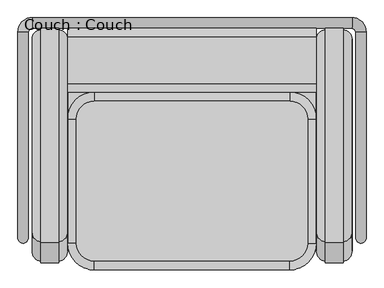
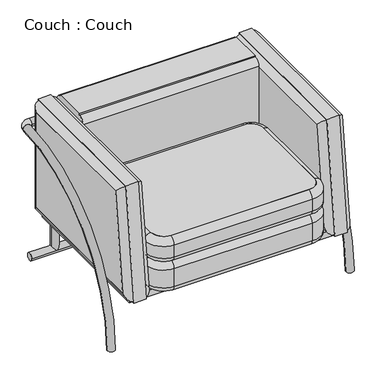
"""IFC4 building model written with IfcOpenShell, lengths in millimetres: furniture geometry, Couch : Couch."""

from ifc_helpers import new_model, si_unit, point, frame, frame_2d, origin, place, context, project, spatial, polyline, circle_curve, ellipse_curve, trimmed, segment, composite_curve, outline, extrude, source, transform, mapped, element, save
from ifc_brep_helpers import plane_surface, cylinder_surface, revolved_surface, advanced_brep


def couch_couch_04099933(model_context):
    return source(origin(), model_context, "Body", "SolidModel", [
        extrude(outline(composite_curve([segment(trimmed(circle_curve(frame_2d((275.0, 175.0)), 50.0), [point((275.0, 225.0))], [point((325.0, 175.0))], False, "CARTESIAN"), True, "CONTINUOUS"), segment(polyline([(325.0, 175.0), (325.0, -175.0)]), True, "CONTINUOUS"), segment(trimmed(circle_curve(frame_2d((275.0, -175.0)), 50.0), [point((325.0, -175.0))], [point((275.0, -225.0))], False, "CARTESIAN"), True, "CONTINUOUS"), segment(polyline([(275.0, -225.0), (-275.0, -225.0)]), True, "CONTINUOUS"), segment(trimmed(circle_curve(frame_2d((-275.0, -175.0)), 50.0), [point((-275.0, -225.0))], [point((-325.0, -175.0))], False, "CARTESIAN"), True, "CONTINUOUS"), segment(polyline([(-325.0, -175.0), (-325.0, 175.0)]), True, "CONTINUOUS"), segment(trimmed(circle_curve(frame_2d((-275.0, 175.0)), 50.0), [point((-325.0, 175.0))], [point((-275.0, 225.0))], False, "CARTESIAN"), True, "CONTINUOUS"), segment(polyline([(-275.0, 225.0), (275.0, 225.0)]), True, "CONTINUOUS")], self_intersect=False)), frame((0.0, 0.0, 350.0), z_axis=(0.0, 0.0, 1.0), x_axis=(1.0, 0.0, 0.0)), (0.0, 0.0, 1.0), 100.0),
        advanced_brep(
        [(-275.0, 225.0, 450.0), (-325.0, 175.0, 450.0), (-325.0, 175.0, 350.0), (-275.0, 225.0, 350.0), (-275.0, 250.0, 425.0), (-350.0, 175.0, 425.0), (-275.0, 250.0, 375.0), (-350.0, 175.0, 375.0), (275.0, 225.0, 350.0), (275.0, 225.0, 450.0), (275.0, 250.0, 425.0), (275.0, 250.0, 375.0), (325.0, 175.0, 450.0), (325.0, 175.0, 350.0), (350.0, 175.0, 425.0), (350.0, 175.0, 375.0), (325.0, -175.0, 350.0), (325.0, -175.0, 450.0), (350.0, -175.0, 425.0), (350.0, -175.0, 375.0), (275.0, -225.0, 450.0), (275.0, -225.0, 350.0), (275.0, -250.0, 425.0), (275.0, -250.0, 375.0), (-275.0, -225.0, 350.0), (-275.0, -225.0, 450.0), (-275.0, -250.0, 425.0), (-275.0, -250.0, 375.0), (-325.0, -175.0, 450.0), (-325.0, -175.0, 350.0), (-350.0, -175.0, 425.0), (-350.0, -175.0, 375.0)],
        [
            (0, 1, circle_curve(frame((-275.0, 175.0, 450.0), z_axis=(0.0, 0.0, 1.0), x_axis=(-1.0, 0.0, 0.0)), 50.0)),
            (1, 2),
            (2, 3, circle_curve(frame((-275.0, 175.0, 350.0), z_axis=(0.0, 0.0, -1.0), x_axis=(-1.0, 0.0, 0.0)), 50.0)),
            (3, 0),
            (4, 5, circle_curve(frame((-275.0, 175.0, 425.0), z_axis=(0.0, 0.0, 1.0), x_axis=(-1.0, 0.0, 0.0)), 75.0)),
            (5, 1, circle_curve(frame((-325.0, 175.0, 425.0), z_axis=(0.0, 1.0, 0.0), x_axis=(1.0, 0.0, 0.0)), 25.0)),
            (0, 4, circle_curve(frame((-275.0, 225.0, 425.0), z_axis=(-1.0, 0.0, 0.0), x_axis=(0.0, -1.0, 0.0)), 25.0)),
            (6, 7, circle_curve(frame((-275.0, 175.0, 375.0), z_axis=(0.0, 0.0, 1.0), x_axis=(-1.0, 0.0, 0.0)), 75.0)),
            (7, 5),
            (4, 6),
            (2, 7, circle_curve(frame((-325.0, 175.0, 375.0), z_axis=(0.0, 1.0, 0.0), x_axis=(1.0, 0.0, 0.0)), 25.0)),
            (6, 3, circle_curve(frame((-275.0, 225.0, 375.0), z_axis=(-1.0, 0.0, 0.0), x_axis=(0.0, -1.0, 0.0)), 25.0)),
            (3, 8),
            (8, 9),
            (9, 0),
            (9, 10, circle_curve(frame((275.0, 225.0, 425.0), z_axis=(-1.0, 0.0, 0.0), x_axis=(0.0, -1.0, 0.0)), 25.0)),
            (10, 4),
            (10, 11),
            (11, 6),
            (11, 8, circle_curve(frame((275.0, 225.0, 375.0), z_axis=(-1.0, 0.0, 0.0), x_axis=(0.0, -1.0, 0.0)), 25.0)),
            (12, 9, circle_curve(frame((275.0, 175.0, 450.0), z_axis=(0.0, 0.0, 1.0), x_axis=(0.0, 1.0, 0.0)), 50.0)),
            (8, 13, circle_curve(frame((275.0, 175.0, 350.0), z_axis=(0.0, 0.0, -1.0), x_axis=(0.0, 1.0, 0.0)), 50.0)),
            (13, 12),
            (14, 10, circle_curve(frame((275.0, 175.0, 425.0), z_axis=(0.0, 0.0, 1.0), x_axis=(0.0, 1.0, 0.0)), 75.0)),
            (12, 14, circle_curve(frame((325.0, 175.0, 425.0), z_axis=(0.0, 1.0, 0.0), x_axis=(-1.0, 0.0, 0.0)), 25.0)),
            (15, 11, circle_curve(frame((275.0, 175.0, 375.0), z_axis=(0.0, 0.0, 1.0), x_axis=(0.0, 1.0, 0.0)), 75.0)),
            (14, 15),
            (15, 13, circle_curve(frame((325.0, 175.0, 375.0), z_axis=(0.0, 1.0, 0.0), x_axis=(-1.0, 0.0, 0.0)), 25.0)),
            (13, 16),
            (16, 17),
            (17, 12),
            (17, 18, circle_curve(frame((325.0, -175.0, 425.0), z_axis=(0.0, 1.0, 0.0), x_axis=(-1.0, 0.0, 0.0)), 25.0)),
            (18, 14),
            (18, 19),
            (19, 15),
            (19, 16, circle_curve(frame((325.0, -175.0, 375.0), z_axis=(0.0, 1.0, 0.0), x_axis=(-1.0, 0.0, 0.0)), 25.0)),
            (20, 17, circle_curve(frame((275.0, -175.0, 450.0), z_axis=(0.0, 0.0, 1.0), x_axis=(1.0, 0.0, 0.0)), 50.0)),
            (16, 21, circle_curve(frame((275.0, -175.0, 350.0), z_axis=(0.0, 0.0, -1.0), x_axis=(1.0, 0.0, 0.0)), 50.0)),
            (21, 20),
            (22, 18, circle_curve(frame((275.0, -175.0, 425.0), z_axis=(0.0, 0.0, 1.0), x_axis=(1.0, 0.0, 0.0)), 75.0)),
            (20, 22, circle_curve(frame((275.0, -225.0, 425.0), z_axis=(1.0, 0.0, 0.0), x_axis=(0.0, 1.0, 0.0)), 25.0)),
            (23, 19, circle_curve(frame((275.0, -175.0, 375.0), z_axis=(0.0, 0.0, 1.0), x_axis=(1.0, 0.0, 0.0)), 75.0)),
            (22, 23),
            (23, 21, circle_curve(frame((275.0, -225.0, 375.0), z_axis=(1.0, 0.0, 0.0), x_axis=(0.0, 1.0, 0.0)), 25.0)),
            (21, 24),
            (24, 25),
            (25, 20),
            (25, 26, circle_curve(frame((-275.0, -225.0, 425.0), z_axis=(1.0, 0.0, 0.0), x_axis=(0.0, 1.0, 0.0)), 25.0)),
            (26, 22),
            (26, 27),
            (27, 23),
            (27, 24, circle_curve(frame((-275.0, -225.0, 375.0), z_axis=(1.0, 0.0, 0.0), x_axis=(0.0, 1.0, 0.0)), 25.0)),
            (28, 25, circle_curve(frame((-275.0, -175.0, 450.0), z_axis=(0.0, 0.0, 1.0), x_axis=(0.0, -1.0, 0.0)), 50.0)),
            (24, 29, circle_curve(frame((-275.0, -175.0, 350.0), z_axis=(0.0, 0.0, -1.0), x_axis=(0.0, -1.0, 0.0)), 50.0)),
            (29, 28),
            (30, 26, circle_curve(frame((-275.0, -175.0, 425.0), z_axis=(0.0, 0.0, 1.0), x_axis=(0.0, -1.0, 0.0)), 75.0)),
            (28, 30, circle_curve(frame((-325.0, -175.0, 425.0), z_axis=(0.0, -1.0, 0.0), x_axis=(1.0, 0.0, 0.0)), 25.0)),
            (31, 27, circle_curve(frame((-275.0, -175.0, 375.0), z_axis=(0.0, 0.0, 1.0), x_axis=(0.0, -1.0, 0.0)), 75.0)),
            (30, 31),
            (31, 29, circle_curve(frame((-325.0, -175.0, 375.0), z_axis=(0.0, -1.0, 0.0), x_axis=(1.0, 0.0, 0.0)), 25.0)),
            (29, 2),
            (1, 28),
            (5, 30),
            (7, 31),
        ],
        [
            revolved_surface(polyline([(-325.0, 175.0, 350.0), (-325.0, 175.0, 450.0)]), (-275.0, 175.0, 0.0), (0.0, 0.0, -1.0)),
            revolved_surface(trimmed(ellipse_curve(frame((-325.0, 175.0, 425.0), z_axis=(0.0, -1.0, 0.0), x_axis=(1.0, 0.0, 0.0)), 25.0, 25.0), [point((-325.0, 175.0, 450.0))], [point((-350.0, 175.0, 425.0))], True, "CARTESIAN"), (-275.0, 175.0, 0.0), (0.0, 0.0, -1.0)),
            cylinder_surface(frame((-275.0, 175.0, 0.0), z_axis=(0.0, 0.0, -1.0), x_axis=(-1.0, 0.0, 0.0)), 75.0),
            revolved_surface(trimmed(ellipse_curve(frame((-325.0, 175.0, 375.0), z_axis=(0.0, -1.0, 0.0), x_axis=(1.0, 0.0, 0.0)), 25.0, 25.0), [point((-350.0, 175.0, 375.0))], [point((-325.0, 175.0, 350.0))], True, "CARTESIAN"), (-275.0, 175.0, 0.0), (0.0, 0.0, -1.0)),
            plane_surface(frame((-275.0, 225.0, 350.0), z_axis=(0.0, -1.0, 0.0), x_axis=(1.0, 0.0, 0.0))),
            cylinder_surface(frame((-275.0, 225.0, 425.0), z_axis=(-1.0, 0.0, 0.0), x_axis=(0.0, -1.0, 0.0)), 25.0),
            plane_surface(frame((-275.0, 250.0, 425.0), z_axis=(0.0, 1.0, 0.0), x_axis=(1.0, 0.0, 0.0))),
            cylinder_surface(frame((-275.0, 225.0, 375.0), z_axis=(-1.0, 0.0, 0.0), x_axis=(0.0, -1.0, 0.0)), 25.0),
            revolved_surface(polyline([(275.0, 225.0, 350.0), (275.0, 225.0, 450.0)]), (275.0, 175.0, 0.0), (0.0, 0.0, -1.0)),
            revolved_surface(trimmed(ellipse_curve(frame((275.0, 225.0, 425.0), z_axis=(-1.0, 0.0, 0.0), x_axis=(0.0, -1.0, 0.0)), 25.0, 25.0), [point((275.0, 225.0, 450.0))], [point((275.0, 250.0, 425.0))], True, "CARTESIAN"), (275.0, 175.0, 0.0), (0.0, 0.0, -1.0)),
            cylinder_surface(frame((275.0, 175.0, 0.0), z_axis=(0.0, 0.0, -1.0), x_axis=(0.0, 1.0, 0.0)), 75.0),
            revolved_surface(trimmed(ellipse_curve(frame((275.0, 225.0, 375.0), z_axis=(-1.0, 0.0, 0.0), x_axis=(0.0, -1.0, 0.0)), 25.0, 25.0), [point((275.0, 250.0, 375.0))], [point((275.0, 225.0, 350.0))], True, "CARTESIAN"), (275.0, 175.0, 0.0), (0.0, 0.0, -1.0)),
            plane_surface(frame((325.0, 175.0, 350.0), z_axis=(-1.0, 0.0, 0.0), x_axis=(0.0, -1.0, 0.0))),
            cylinder_surface(frame((325.0, 175.0, 425.0), z_axis=(0.0, 1.0, 0.0), x_axis=(-1.0, 0.0, 0.0)), 25.0),
            plane_surface(frame((350.0, 175.0, 425.0), z_axis=(1.0, 0.0, 0.0), x_axis=(0.0, -1.0, 0.0))),
            cylinder_surface(frame((325.0, 175.0, 375.0), z_axis=(0.0, 1.0, 0.0), x_axis=(-1.0, 0.0, 0.0)), 25.0),
            revolved_surface(polyline([(325.0, -175.0, 350.0), (325.0, -175.0, 450.0)]), (275.0, -175.0, 0.0), (0.0, 0.0, -1.0)),
            revolved_surface(trimmed(ellipse_curve(frame((325.0, -175.0, 425.0), z_axis=(0.0, 1.0, 0.0), x_axis=(-1.0, 0.0, 0.0)), 25.0, 25.0), [point((325.0, -175.0, 450.0))], [point((350.0, -175.0, 425.0))], True, "CARTESIAN"), (275.0, -175.0, 0.0), (0.0, 0.0, -1.0)),
            cylinder_surface(frame((275.0, -175.0, 0.0), z_axis=(0.0, 0.0, -1.0), x_axis=(1.0, 0.0, 0.0)), 75.0),
            revolved_surface(trimmed(ellipse_curve(frame((325.0, -175.0, 375.0), z_axis=(0.0, 1.0, 0.0), x_axis=(-1.0, 0.0, 0.0)), 25.0, 25.0), [point((350.0, -175.0, 375.0))], [point((325.0, -175.0, 350.0))], True, "CARTESIAN"), (275.0, -175.0, 0.0), (0.0, 0.0, -1.0)),
            plane_surface(frame((275.0, -225.0, 350.0), z_axis=(0.0, 1.0, 0.0), x_axis=(-1.0, 0.0, 0.0))),
            cylinder_surface(frame((275.0, -225.0, 425.0), z_axis=(1.0, 0.0, 0.0), x_axis=(0.0, 1.0, 0.0)), 25.0),
            plane_surface(frame((275.0, -250.0, 425.0), z_axis=(0.0, -1.0, 0.0), x_axis=(-1.0, 0.0, 0.0))),
            cylinder_surface(frame((275.0, -225.0, 375.0), z_axis=(1.0, 0.0, 0.0), x_axis=(0.0, 1.0, 0.0)), 25.0),
            revolved_surface(polyline([(-275.0, -225.0, 350.0), (-275.0, -225.0, 450.0)]), (-275.0, -175.0, 0.0), (0.0, 0.0, -1.0)),
            revolved_surface(trimmed(ellipse_curve(frame((-275.0, -225.0, 425.0), z_axis=(1.0, 0.0, 0.0), x_axis=(0.0, 1.0, 0.0)), 25.0, 25.0), [point((-275.0, -225.0, 450.0))], [point((-275.0, -250.0, 425.0))], True, "CARTESIAN"), (-275.0, -175.0, 0.0), (0.0, 0.0, -1.0)),
            cylinder_surface(frame((-275.0, -175.0, 0.0), z_axis=(0.0, 0.0, -1.0), x_axis=(0.0, -1.0, 0.0)), 75.0),
            revolved_surface(trimmed(ellipse_curve(frame((-275.0, -225.0, 375.0), z_axis=(1.0, 0.0, 0.0), x_axis=(0.0, 1.0, 0.0)), 25.0, 25.0), [point((-275.0, -250.0, 375.0))], [point((-275.0, -225.0, 350.0))], True, "CARTESIAN"), (-275.0, -175.0, 0.0), (0.0, 0.0, -1.0)),
            plane_surface(frame((-325.0, -175.0, 350.0), z_axis=(1.0, 0.0, 0.0), x_axis=(0.0, 1.0, 0.0))),
            cylinder_surface(frame((-325.0, -175.0, 425.0), z_axis=(0.0, -1.0, 0.0), x_axis=(1.0, 0.0, 0.0)), 25.0),
            plane_surface(frame((-350.0, -175.0, 425.0), z_axis=(-1.0, 0.0, 0.0), x_axis=(0.0, 1.0, 0.0))),
            cylinder_surface(frame((-325.0, -175.0, 375.0), z_axis=(0.0, -1.0, 0.0), x_axis=(1.0, 0.0, 0.0)), 25.0),
        ],
        [
            (0, [[1, 2, 3, 4]]),
            (1, [[5, 6, -1, 7]]),
            (2, [[8, 9, -5, 10]]),
            (3, [[-3, 11, -8, 12]]),
            (4, [[-4, 13, 14, 15]]),
            (5, [[-7, -15, 16, 17]]),
            (6, [[-10, -17, 18, 19]]),
            (7, [[-12, -19, 20, -13]]),
            (8, [[21, -14, 22, 23]]),
            (9, [[24, -16, -21, 25]]),
            (10, [[26, -18, -24, 27]]),
            (11, [[-22, -20, -26, 28]]),
            (12, [[-23, 29, 30, 31]]),
            (13, [[-25, -31, 32, 33]]),
            (14, [[-27, -33, 34, 35]]),
            (15, [[-28, -35, 36, -29]]),
            (16, [[37, -30, 38, 39]]),
            (17, [[40, -32, -37, 41]]),
            (18, [[42, -34, -40, 43]]),
            (19, [[-38, -36, -42, 44]]),
            (20, [[-39, 45, 46, 47]]),
            (21, [[-41, -47, 48, 49]]),
            (22, [[-43, -49, 50, 51]]),
            (23, [[-44, -51, 52, -45]]),
            (24, [[53, -46, 54, 55]]),
            (25, [[56, -48, -53, 57]]),
            (26, [[58, -50, -56, 59]]),
            (27, [[-54, -52, -58, 60]]),
            (28, [[-55, 61, -2, 62]]),
            (29, [[-57, -62, -6, 63]]),
            (30, [[-59, -63, -9, 64]]),
            (31, [[-60, -64, -11, -61]]),
        ],
    ),
        advanced_brep(
        [(-275.0, 225.0, 350.0), (-325.0, 175.0, 350.0), (-325.0, 175.0, 225.0), (-275.0, 225.0, 225.0), (-275.0, 250.0, 325.0), (-350.0, 175.0, 325.0), (-275.0, 250.0, 250.0), (-350.0, 175.0, 250.0), (275.0, 225.0, 225.0), (275.0, 225.0, 350.0), (275.0, 250.0, 325.0), (275.0, 250.0, 250.0), (325.0, 175.0, 350.0), (325.0, 175.0, 225.0), (350.0, 175.0, 325.0), (350.0, 175.0, 250.0), (325.0, -175.0, 225.0), (325.0, -175.0, 350.0), (350.0, -175.0, 325.0), (350.0, -175.0, 250.0), (275.0, -225.0, 350.0), (275.0, -225.0, 225.0), (275.0, -250.0, 325.0), (275.0, -250.0, 250.0), (-275.0, -225.0, 225.0), (-275.0, -225.0, 350.0), (-275.0, -250.0, 325.0), (-275.0, -250.0, 250.0), (-325.0, -175.0, 350.0), (-325.0, -175.0, 225.0), (-350.0, -175.0, 325.0), (-350.0, -175.0, 250.0)],
        [
            (0, 1, circle_curve(frame((-275.0, 175.0, 350.0), z_axis=(0.0, 0.0, 1.0), x_axis=(-1.0, 0.0, 0.0)), 50.0)),
            (1, 2),
            (2, 3, circle_curve(frame((-275.0, 175.0, 225.0), z_axis=(0.0, 0.0, -1.0), x_axis=(-1.0, 0.0, 0.0)), 50.0)),
            (3, 0),
            (4, 5, circle_curve(frame((-275.0, 175.0, 325.0), z_axis=(0.0, 0.0, 1.0), x_axis=(-1.0, 0.0, 0.0)), 75.0)),
            (5, 1, circle_curve(frame((-325.0, 175.0, 325.0), z_axis=(0.0, 1.0, 0.0), x_axis=(1.0, 0.0, 0.0)), 25.0)),
            (0, 4, circle_curve(frame((-275.0, 225.0, 325.0), z_axis=(-1.0, 0.0, 0.0), x_axis=(0.0, -1.0, 0.0)), 25.0)),
            (6, 7, circle_curve(frame((-275.0, 175.0, 250.0), z_axis=(0.0, 0.0, 1.0), x_axis=(-1.0, 0.0, 0.0)), 75.0)),
            (7, 5),
            (4, 6),
            (2, 7, circle_curve(frame((-325.0, 175.0, 250.0), z_axis=(0.0, 1.0, 0.0), x_axis=(1.0, 0.0, 0.0)), 25.0)),
            (6, 3, circle_curve(frame((-275.0, 225.0, 250.0), z_axis=(-1.0, 0.0, 0.0), x_axis=(0.0, -1.0, 0.0)), 25.0)),
            (3, 8),
            (8, 9),
            (9, 0),
            (9, 10, circle_curve(frame((275.0, 225.0, 325.0), z_axis=(-1.0, 0.0, 0.0), x_axis=(0.0, -1.0, 0.0)), 25.0)),
            (10, 4),
            (10, 11),
            (11, 6),
            (11, 8, circle_curve(frame((275.0, 225.0, 250.0), z_axis=(-1.0, 0.0, 0.0), x_axis=(0.0, -1.0, 0.0)), 25.0)),
            (12, 9, circle_curve(frame((275.0, 175.0, 350.0), z_axis=(0.0, 0.0, 1.0), x_axis=(0.0, 1.0, 0.0)), 50.0)),
            (8, 13, circle_curve(frame((275.0, 175.0, 225.0), z_axis=(0.0, 0.0, -1.0), x_axis=(0.0, 1.0, 0.0)), 50.0)),
            (13, 12),
            (14, 10, circle_curve(frame((275.0, 175.0, 325.0), z_axis=(0.0, 0.0, 1.0), x_axis=(0.0, 1.0, 0.0)), 75.0)),
            (12, 14, circle_curve(frame((325.0, 175.0, 325.0), z_axis=(0.0, 1.0, 0.0), x_axis=(-1.0, 0.0, 0.0)), 25.0)),
            (15, 11, circle_curve(frame((275.0, 175.0, 250.0), z_axis=(0.0, 0.0, 1.0), x_axis=(0.0, 1.0, 0.0)), 75.0)),
            (14, 15),
            (15, 13, circle_curve(frame((325.0, 175.0, 250.0), z_axis=(0.0, 1.0, 0.0), x_axis=(-1.0, 0.0, 0.0)), 25.0)),
            (13, 16),
            (16, 17),
            (17, 12),
            (17, 18, circle_curve(frame((325.0, -175.0, 325.0), z_axis=(0.0, 1.0, 0.0), x_axis=(-1.0, 0.0, 0.0)), 25.0)),
            (18, 14),
            (18, 19),
            (19, 15),
            (19, 16, circle_curve(frame((325.0, -175.0, 250.0), z_axis=(0.0, 1.0, 0.0), x_axis=(-1.0, 0.0, 0.0)), 25.0)),
            (20, 17, circle_curve(frame((275.0, -175.0, 350.0), z_axis=(0.0, 0.0, 1.0), x_axis=(1.0, 0.0, 0.0)), 50.0)),
            (16, 21, circle_curve(frame((275.0, -175.0, 225.0), z_axis=(0.0, 0.0, -1.0), x_axis=(1.0, 0.0, 0.0)), 50.0)),
            (21, 20),
            (22, 18, circle_curve(frame((275.0, -175.0, 325.0), z_axis=(0.0, 0.0, 1.0), x_axis=(1.0, 0.0, 0.0)), 75.0)),
            (20, 22, circle_curve(frame((275.0, -225.0, 325.0), z_axis=(1.0, 0.0, 0.0), x_axis=(0.0, 1.0, 0.0)), 25.0)),
            (23, 19, circle_curve(frame((275.0, -175.0, 250.0), z_axis=(0.0, 0.0, 1.0), x_axis=(1.0, 0.0, 0.0)), 75.0)),
            (22, 23),
            (23, 21, circle_curve(frame((275.0, -225.0, 250.0), z_axis=(1.0, 0.0, 0.0), x_axis=(0.0, 1.0, 0.0)), 25.0)),
            (21, 24),
            (24, 25),
            (25, 20),
            (25, 26, circle_curve(frame((-275.0, -225.0, 325.0), z_axis=(1.0, 0.0, 0.0), x_axis=(0.0, 1.0, 0.0)), 25.0)),
            (26, 22),
            (26, 27),
            (27, 23),
            (27, 24, circle_curve(frame((-275.0, -225.0, 250.0), z_axis=(1.0, 0.0, 0.0), x_axis=(0.0, 1.0, 0.0)), 25.0)),
            (28, 25, circle_curve(frame((-275.0, -175.0, 350.0), z_axis=(0.0, 0.0, 1.0), x_axis=(0.0, -1.0, 0.0)), 50.0)),
            (24, 29, circle_curve(frame((-275.0, -175.0, 225.0), z_axis=(0.0, 0.0, -1.0), x_axis=(0.0, -1.0, 0.0)), 50.0)),
            (29, 28),
            (30, 26, circle_curve(frame((-275.0, -175.0, 325.0), z_axis=(0.0, 0.0, 1.0), x_axis=(0.0, -1.0, 0.0)), 75.0)),
            (28, 30, circle_curve(frame((-325.0, -175.0, 325.0), z_axis=(0.0, -1.0, 0.0), x_axis=(1.0, 0.0, 0.0)), 25.0)),
            (31, 27, circle_curve(frame((-275.0, -175.0, 250.0), z_axis=(0.0, 0.0, 1.0), x_axis=(0.0, -1.0, 0.0)), 75.0)),
            (30, 31),
            (31, 29, circle_curve(frame((-325.0, -175.0, 250.0), z_axis=(0.0, -1.0, 0.0), x_axis=(1.0, 0.0, 0.0)), 25.0)),
            (29, 2),
            (1, 28),
            (5, 30),
            (7, 31),
        ],
        [
            revolved_surface(polyline([(-325.0, 175.0, 225.0), (-325.0, 175.0, 350.0)]), (-275.0, 175.0, -75.0), (0.0, 0.0, -1.0)),
            revolved_surface(trimmed(ellipse_curve(frame((-325.0, 175.0, 325.0), z_axis=(0.0, -1.0, 0.0), x_axis=(1.0, 0.0, 0.0)), 25.0, 25.0), [point((-325.0, 175.0, 350.0))], [point((-350.0, 175.0, 325.0))], True, "CARTESIAN"), (-275.0, 175.0, -75.0), (0.0, 0.0, -1.0)),
            cylinder_surface(frame((-275.0, 175.0, -75.0), z_axis=(0.0, 0.0, -1.0), x_axis=(-1.0, 0.0, 0.0)), 75.0),
            revolved_surface(trimmed(ellipse_curve(frame((-325.0, 175.0, 250.0), z_axis=(0.0, -1.0, 0.0), x_axis=(1.0, 0.0, 0.0)), 25.0, 25.0), [point((-350.0, 175.0, 250.0))], [point((-325.0, 175.0, 225.0))], True, "CARTESIAN"), (-275.0, 175.0, -75.0), (0.0, 0.0, -1.0)),
            plane_surface(frame((-275.0, 225.0, 225.0), z_axis=(0.0, -1.0, 0.0), x_axis=(1.0, 0.0, 0.0))),
            cylinder_surface(frame((-275.0, 225.0, 325.0), z_axis=(-1.0, 0.0, 0.0), x_axis=(0.0, -1.0, 0.0)), 25.0),
            plane_surface(frame((-275.0, 250.0, 325.0), z_axis=(0.0, 1.0, 0.0), x_axis=(1.0, 0.0, 0.0))),
            cylinder_surface(frame((-275.0, 225.0, 250.0), z_axis=(-1.0, 0.0, 0.0), x_axis=(0.0, -1.0, 0.0)), 25.0),
            revolved_surface(polyline([(275.0, 225.0, 225.0), (275.0, 225.0, 350.0)]), (275.0, 175.0, -75.0), (0.0, 0.0, -1.0)),
            revolved_surface(trimmed(ellipse_curve(frame((275.0, 225.0, 325.0), z_axis=(-1.0, 0.0, 0.0), x_axis=(0.0, -1.0, 0.0)), 25.0, 25.0), [point((275.0, 225.0, 350.0))], [point((275.0, 250.0, 325.0))], True, "CARTESIAN"), (275.0, 175.0, -75.0), (0.0, 0.0, -1.0)),
            cylinder_surface(frame((275.0, 175.0, -75.0), z_axis=(0.0, 0.0, -1.0), x_axis=(0.0, 1.0, 0.0)), 75.0),
            revolved_surface(trimmed(ellipse_curve(frame((275.0, 225.0, 250.0), z_axis=(-1.0, 0.0, 0.0), x_axis=(0.0, -1.0, 0.0)), 25.0, 25.0), [point((275.0, 250.0, 250.0))], [point((275.0, 225.0, 225.0))], True, "CARTESIAN"), (275.0, 175.0, -75.0), (0.0, 0.0, -1.0)),
            plane_surface(frame((325.0, 175.0, 225.0), z_axis=(-1.0, 0.0, 0.0), x_axis=(0.0, -1.0, 0.0))),
            cylinder_surface(frame((325.0, 175.0, 325.0), z_axis=(0.0, 1.0, 0.0), x_axis=(-1.0, 0.0, 0.0)), 25.0),
            plane_surface(frame((350.0, 175.0, 325.0), z_axis=(1.0, 0.0, 0.0), x_axis=(0.0, -1.0, 0.0))),
            cylinder_surface(frame((325.0, 175.0, 250.0), z_axis=(0.0, 1.0, 0.0), x_axis=(-1.0, 0.0, 0.0)), 25.0),
            revolved_surface(polyline([(325.0, -175.0, 225.0), (325.0, -175.0, 350.0)]), (275.0, -175.0, -75.0), (0.0, 0.0, -1.0)),
            revolved_surface(trimmed(ellipse_curve(frame((325.0, -175.0, 325.0), z_axis=(0.0, 1.0, 0.0), x_axis=(-1.0, 0.0, 0.0)), 25.0, 25.0), [point((325.0, -175.0, 350.0))], [point((350.0, -175.0, 325.0))], True, "CARTESIAN"), (275.0, -175.0, -75.0), (0.0, 0.0, -1.0)),
            cylinder_surface(frame((275.0, -175.0, -75.0), z_axis=(0.0, 0.0, -1.0), x_axis=(1.0, 0.0, 0.0)), 75.0),
            revolved_surface(trimmed(ellipse_curve(frame((325.0, -175.0, 250.0), z_axis=(0.0, 1.0, 0.0), x_axis=(-1.0, 0.0, 0.0)), 25.0, 25.0), [point((350.0, -175.0, 250.0))], [point((325.0, -175.0, 225.0))], True, "CARTESIAN"), (275.0, -175.0, -75.0), (0.0, 0.0, -1.0)),
            plane_surface(frame((275.0, -225.0, 225.0), z_axis=(0.0, 1.0, 0.0), x_axis=(-1.0, 0.0, 0.0))),
            cylinder_surface(frame((275.0, -225.0, 325.0), z_axis=(1.0, 0.0, 0.0), x_axis=(0.0, 1.0, 0.0)), 25.0),
            plane_surface(frame((275.0, -250.0, 325.0), z_axis=(0.0, -1.0, 0.0), x_axis=(-1.0, 0.0, 0.0))),
            cylinder_surface(frame((275.0, -225.0, 250.0), z_axis=(1.0, 0.0, 0.0), x_axis=(0.0, 1.0, 0.0)), 25.0),
            revolved_surface(polyline([(-275.0, -225.0, 225.0), (-275.0, -225.0, 350.0)]), (-275.0, -175.0, -75.0), (0.0, 0.0, -1.0)),
            revolved_surface(trimmed(ellipse_curve(frame((-275.0, -225.0, 325.0), z_axis=(1.0, 0.0, 0.0), x_axis=(0.0, 1.0, 0.0)), 25.0, 25.0), [point((-275.0, -225.0, 350.0))], [point((-275.0, -250.0, 325.0))], True, "CARTESIAN"), (-275.0, -175.0, -75.0), (0.0, 0.0, -1.0)),
            cylinder_surface(frame((-275.0, -175.0, -75.0), z_axis=(0.0, 0.0, -1.0), x_axis=(0.0, -1.0, 0.0)), 75.0),
            revolved_surface(trimmed(ellipse_curve(frame((-275.0, -225.0, 250.0), z_axis=(1.0, 0.0, 0.0), x_axis=(0.0, 1.0, 0.0)), 25.0, 25.0), [point((-275.0, -250.0, 250.0))], [point((-275.0, -225.0, 225.0))], True, "CARTESIAN"), (-275.0, -175.0, -75.0), (0.0, 0.0, -1.0)),
            plane_surface(frame((-325.0, -175.0, 225.0), z_axis=(1.0, 0.0, 0.0), x_axis=(0.0, 1.0, 0.0))),
            cylinder_surface(frame((-325.0, -175.0, 325.0), z_axis=(0.0, -1.0, 0.0), x_axis=(1.0, 0.0, 0.0)), 25.0),
            plane_surface(frame((-350.0, -175.0, 325.0), z_axis=(-1.0, 0.0, 0.0), x_axis=(0.0, 1.0, 0.0))),
            cylinder_surface(frame((-325.0, -175.0, 250.0), z_axis=(0.0, -1.0, 0.0), x_axis=(1.0, 0.0, 0.0)), 25.0),
        ],
        [
            (0, [[1, 2, 3, 4]]),
            (1, [[5, 6, -1, 7]]),
            (2, [[8, 9, -5, 10]]),
            (3, [[-3, 11, -8, 12]]),
            (4, [[-4, 13, 14, 15]]),
            (5, [[-7, -15, 16, 17]]),
            (6, [[-10, -17, 18, 19]]),
            (7, [[-12, -19, 20, -13]]),
            (8, [[21, -14, 22, 23]]),
            (9, [[24, -16, -21, 25]]),
            (10, [[26, -18, -24, 27]]),
            (11, [[-22, -20, -26, 28]]),
            (12, [[-23, 29, 30, 31]]),
            (13, [[-25, -31, 32, 33]]),
            (14, [[-27, -33, 34, 35]]),
            (15, [[-28, -35, 36, -29]]),
            (16, [[37, -30, 38, 39]]),
            (17, [[40, -32, -37, 41]]),
            (18, [[42, -34, -40, 43]]),
            (19, [[-38, -36, -42, 44]]),
            (20, [[-39, 45, 46, 47]]),
            (21, [[-41, -47, 48, 49]]),
            (22, [[-43, -49, 50, 51]]),
            (23, [[-44, -51, 52, -45]]),
            (24, [[53, -46, 54, 55]]),
            (25, [[56, -48, -53, 57]]),
            (26, [[58, -50, -56, 59]]),
            (27, [[-54, -52, -58, 60]]),
            (28, [[-55, 61, -2, 62]]),
            (29, [[-57, -62, -6, 63]]),
            (30, [[-59, -63, -9, 64]]),
            (31, [[-60, -64, -11, -61]]),
        ],
    ),
        extrude(outline(composite_curve([segment(trimmed(circle_curve(frame_2d((275.0, 175.0)), 50.0), [point((275.0, 225.0))], [point((325.0, 175.0))], False, "CARTESIAN"), True, "CONTINUOUS"), segment(polyline([(325.0, 175.0), (325.0, -175.0)]), True, "CONTINUOUS"), segment(trimmed(circle_curve(frame_2d((275.0, -175.0)), 50.0), [point((325.0, -175.0))], [point((275.0, -225.0))], False, "CARTESIAN"), True, "CONTINUOUS"), segment(polyline([(275.0, -225.0), (-275.0, -225.0)]), True, "CONTINUOUS"), segment(trimmed(circle_curve(frame_2d((-275.0, -175.0)), 50.0), [point((-275.0, -225.0))], [point((-325.0, -175.0))], False, "CARTESIAN"), True, "CONTINUOUS"), segment(polyline([(-325.0, -175.0), (-325.0, 175.0)]), True, "CONTINUOUS"), segment(trimmed(circle_curve(frame_2d((-275.0, 175.0)), 50.0), [point((-325.0, 175.0))], [point((-275.0, 225.0))], False, "CARTESIAN"), True, "CONTINUOUS"), segment(polyline([(-275.0, 225.0), (275.0, 225.0)]), True, "CONTINUOUS")], self_intersect=False)), frame((0.0, 0.0, 225.0), z_axis=(0.0, 0.0, 1.0), x_axis=(1.0, 0.0, 0.0)), (0.0, 0.0, 1.0), 125.0),
        extrude(outline(polyline([(-147.628816, 650.0), (400.0, 650.0), (400.0, 250.0), (-196.7426403, 250.0), (-147.628816, 650.0)])), frame((350.0, 0.0, 0.0), z_axis=(1.0, 0.0, 0.0), x_axis=(0.0, 1.0, 0.0)), (0.0, 0.0, 1.0), 100.0),
        advanced_brep(
        [(450.0, 400.0, 650.0), (350.0, 400.0, 650.0), (350.0, 400.0, 250.0), (450.0, 400.0, 250.0), (425.0, 425.0, 675.0), (425.0, 425.0, 225.0), (375.0, 430.0, 680.0), (425.0, 430.0, 680.0), (425.0, 430.0, 220.0), (375.0, 430.0, 220.0), (375.0, 425.0, 675.0), (375.0, 425.0, 225.0), (350.0, -196.7426403, 250.0), (450.0, -196.7426403, 250.0), (425.0, -225.0, 225.0), (425.0, -230.6514719, 220.0), (375.0, -230.6514719, 220.0), (375.0, -225.0, 225.0), (350.0, -147.628816, 650.0), (450.0, -147.628816, 650.0), (425.0, -169.7469476, 675.0), (425.0, -174.1705739, 680.0), (375.0, -174.1705739, 680.0), (375.0, -169.7469476, 675.0)],
        [
            (0, 1),
            (1, 2),
            (2, 3),
            (3, 0),
            (4, 0, ellipse_curve(frame((425.0, 400.0, 650.0), z_axis=(0.0, 0.7071067811865459, -0.7071067811865492), x_axis=(0.0, 0.7071067811865492, 0.7071067811865458)), 35.3553391, 25.0)),
            (3, 5, ellipse_curve(frame((425.0, 400.0, 250.0), z_axis=(0.0, 0.707106781186549, 0.7071067811865459), x_axis=(0.0, -0.7071067811865458, 0.7071067811865491)), 35.3553391, 25.0)),
            (5, 4),
            (6, 7),
            (7, 8),
            (8, 9),
            (9, 6),
            (1, 10, ellipse_curve(frame((375.0, 400.0, 650.0), z_axis=(0.0, 0.7071067811865459, -0.7071067811865492), x_axis=(0.0, 0.7071067811865492, 0.7071067811865458)), 35.3553391, 25.0)),
            (10, 11),
            (11, 2, ellipse_curve(frame((375.0, 400.0, 250.0), z_axis=(0.0, 0.707106781186549, 0.7071067811865459), x_axis=(0.0, -0.7071067811865458, 0.7071067811865491)), 35.3553391, 25.0)),
            (2, 12),
            (12, 13),
            (13, 3),
            (13, 14, ellipse_curve(frame((425.0, -196.7426403, 250.0), z_axis=(0.0, 0.662620048215735, -0.7489557207890044), x_axis=(0.0, 0.7489557207890045, 0.662620048215735)), 37.7290124, 25.0)),
            (14, 5),
            (8, 15),
            (15, 16),
            (16, 9),
            (11, 17),
            (17, 12, ellipse_curve(frame((375.0, -196.7426403, 250.0), z_axis=(0.0, 0.662620048215735, -0.7489557207890044), x_axis=(0.0, 0.7489557207890045, 0.662620048215735)), 37.7290124, 25.0)),
            (12, 18),
            (18, 19),
            (19, 13),
            (19, 20, ellipse_curve(frame((425.0, -147.628816, 650.0), z_axis=(0.0, -0.7489557207890044, -0.6626200482157351), x_axis=(0.0, 0.6626200482157352, -0.7489557207890042)), 33.3798105, 25.0)),
            (20, 14),
            (15, 21),
            (21, 22),
            (22, 16),
            (17, 23),
            (23, 18, ellipse_curve(frame((375.0, -147.628816, 650.0), z_axis=(0.0, -0.7489557207890044, -0.6626200482157351), x_axis=(0.0, 0.6626200482157352, -0.7489557207890042)), 33.3798105, 25.0)),
            (18, 1),
            (0, 19),
            (4, 20),
            (7, 21),
            (6, 22),
            (10, 23),
        ],
        [
            plane_surface(frame((350.0, 400.0, 650.0), z_axis=(0.0, -1.0, 0.0), x_axis=(0.0, 0.0, -1.0))),
            cylinder_surface(frame((425.0, 400.0, 650.0), z_axis=(0.0, 0.0, 1.0), x_axis=(1.0, 0.0, 0.0)), 25.0),
            plane_surface(frame((425.0, 430.0, 680.0), z_axis=(0.0, 1.0, 0.0), x_axis=(0.0, 0.0, -1.0))),
            cylinder_surface(frame((375.0, 400.0, 650.0), z_axis=(0.0, 0.0, 1.0), x_axis=(-1.0, 0.0, 0.0)), 25.0),
            plane_surface(frame((350.0, 400.0, 250.0), z_axis=(0.0, 0.0, 1.0), x_axis=(0.0, -1.0, 0.0))),
            cylinder_surface(frame((425.0, 400.0, 250.0), z_axis=(0.0, 1.0, 0.0), x_axis=(1.0, 0.0, 0.0)), 25.0),
            plane_surface(frame((425.0, 430.0, 220.0), z_axis=(0.0, 0.0, -1.0), x_axis=(0.0, -1.0, 0.0))),
            cylinder_surface(frame((375.0, 400.0, 250.0), z_axis=(0.0, 1.0, 0.0), x_axis=(-1.0, 0.0, 0.0)), 25.0),
            plane_surface(frame((350.0, -196.7426403, 250.0), z_axis=(0.0, 0.9925461516413217, -0.12186934340515108), x_axis=(0.0, 0.12186934340515108, 0.9925461516413217))),
            cylinder_surface(frame((425.0, -196.7426403, 250.0), z_axis=(0.0, -0.121869343405151, -0.9925461516413215), x_axis=(1.0, 0.0, 0.0)), 25.0),
            plane_surface(frame((425.0, -230.6514719, 220.0), z_axis=(0.0, -0.9925461516413215, 0.12186934340515118), x_axis=(0.0, 0.12186934340515118, 0.9925461516413215))),
            cylinder_surface(frame((375.0, -196.7426403, 250.0), z_axis=(0.0, -0.121869343405151, -0.9925461516413215), x_axis=(-1.0, 0.0, 0.0)), 25.0),
            plane_surface(frame((350.0, -147.628816, 650.0), z_axis=(0.0, 0.0, -1.0), x_axis=(0.0, 1.0, 0.0))),
            cylinder_surface(frame((425.0, -147.628816, 650.0), z_axis=(0.0, -1.0, 0.0), x_axis=(1.0, 0.0, 0.0)), 25.0),
            plane_surface(frame((425.0, -169.7469476, 675.0), z_axis=(1.0, 0.0, 0.0), x_axis=(0.0, 1.0, 0.0))),
            plane_surface(frame((425.0, -174.1705739, 680.0), z_axis=(0.0, 0.0, 1.0), x_axis=(0.0, 1.0, 0.0))),
            plane_surface(frame((375.0, -174.1705739, 680.0), z_axis=(-1.0, 0.0, 0.0), x_axis=(0.0, 1.0, 0.0))),
            cylinder_surface(frame((375.0, -147.628816, 650.0), z_axis=(0.0, -1.0, 0.0), x_axis=(-1.0, 0.0, 0.0)), 25.0),
        ],
        [
            (0, [[1, 2, 3, 4]]),
            (1, [[5, -4, 6, 7]]),
            (2, [[8, 9, 10, 11]]),
            (3, [[12, 13, 14, -2]]),
            (4, [[-3, 15, 16, 17]]),
            (5, [[-6, -17, 18, 19]]),
            (6, [[-10, 20, 21, 22]]),
            (7, [[-14, 23, 24, -15]]),
            (8, [[-16, 25, 26, 27]]),
            (9, [[-18, -27, 28, 29]]),
            (10, [[-21, 30, 31, 32]]),
            (11, [[-24, 33, 34, -25]]),
            (12, [[-26, 35, -1, 36]]),
            (13, [[-28, -36, -5, 37]]),
            (14, [[38, -30, -20, -9], [-19, -29, -37, -7]]),
            (15, [[-31, -38, -8, 39]]),
            (16, [[-22, -32, -39, -11], [40, -33, -23, -13]]),
            (17, [[-34, -40, -12, -35]]),
        ],
    ),
        extrude(outline(polyline([(-147.628816, 650.0), (400.0, 650.0), (400.0, 250.0), (-196.7426403, 250.0), (-147.628816, 650.0)])), frame((-450.0, 0.0, 0.0), z_axis=(1.0, 0.0, 0.0), x_axis=(0.0, 1.0, 0.0)), (0.0, 0.0, 1.0), 100.0),
        advanced_brep(
        [(-350.0, 400.0, 650.0), (-450.0, 400.0, 650.0), (-450.0, 400.0, 250.0), (-350.0, 400.0, 250.0), (-375.0, 425.0, 675.0), (-375.0, 425.0, 225.0), (-425.0, 430.0, 680.0), (-375.0, 430.0, 680.0), (-375.0, 430.0, 220.0), (-425.0, 430.0, 220.0), (-425.0, 425.0, 675.0), (-425.0, 425.0, 225.0), (-450.0, -196.7426403, 250.0), (-350.0, -196.7426403, 250.0), (-375.0, -225.0, 225.0), (-375.0, -230.6514719, 220.0), (-425.0, -230.6514719, 220.0), (-425.0, -225.0, 225.0), (-450.0, -147.628816, 650.0), (-350.0, -147.628816, 650.0), (-375.0, -169.7469476, 675.0), (-375.0, -174.1705739, 680.0), (-425.0, -174.1705739, 680.0), (-425.0, -169.7469476, 675.0)],
        [
            (0, 1),
            (1, 2),
            (2, 3),
            (3, 0),
            (4, 0, ellipse_curve(frame((-375.0, 400.0, 650.0), z_axis=(0.0, 0.7071067811865459, -0.7071067811865492), x_axis=(0.0, 0.7071067811865492, 0.7071067811865458)), 35.3553391, 25.0)),
            (3, 5, ellipse_curve(frame((-375.0, 400.0, 250.0), z_axis=(0.0, 0.707106781186549, 0.7071067811865459), x_axis=(0.0, -0.7071067811865458, 0.7071067811865491)), 35.3553391, 25.0)),
            (5, 4),
            (6, 7),
            (7, 8),
            (8, 9),
            (9, 6),
            (1, 10, ellipse_curve(frame((-425.0, 400.0, 650.0), z_axis=(0.0, 0.7071067811865459, -0.7071067811865492), x_axis=(0.0, 0.7071067811865492, 0.7071067811865458)), 35.3553391, 25.0)),
            (10, 11),
            (11, 2, ellipse_curve(frame((-425.0, 400.0, 250.0), z_axis=(0.0, 0.707106781186549, 0.7071067811865459), x_axis=(0.0, -0.7071067811865458, 0.7071067811865491)), 35.3553391, 25.0)),
            (2, 12),
            (12, 13),
            (13, 3),
            (13, 14, ellipse_curve(frame((-375.0, -196.7426403, 250.0), z_axis=(0.0, 0.662620048215735, -0.7489557207890044), x_axis=(0.0, 0.7489557207890045, 0.662620048215735)), 37.7290124, 25.0)),
            (14, 5),
            (8, 15),
            (15, 16),
            (16, 9),
            (11, 17),
            (17, 12, ellipse_curve(frame((-425.0, -196.7426403, 250.0), z_axis=(0.0, 0.662620048215735, -0.7489557207890044), x_axis=(0.0, 0.7489557207890045, 0.662620048215735)), 37.7290124, 25.0)),
            (12, 18),
            (18, 19),
            (19, 13),
            (19, 20, ellipse_curve(frame((-375.0, -147.628816, 650.0), z_axis=(0.0, -0.7489557207890044, -0.6626200482157351), x_axis=(0.0, 0.6626200482157352, -0.7489557207890042)), 33.3798105, 25.0)),
            (20, 14),
            (15, 21),
            (21, 22),
            (22, 16),
            (17, 23),
            (23, 18, ellipse_curve(frame((-425.0, -147.628816, 650.0), z_axis=(0.0, -0.7489557207890044, -0.6626200482157351), x_axis=(0.0, 0.6626200482157352, -0.7489557207890042)), 33.3798105, 25.0)),
            (18, 1),
            (0, 19),
            (4, 20),
            (7, 21),
            (6, 22),
            (10, 23),
        ],
        [
            plane_surface(frame((-450.0, 400.0, 650.0), z_axis=(0.0, -1.0, 0.0), x_axis=(0.0, 0.0, -1.0))),
            cylinder_surface(frame((-375.0, 400.0, 650.0), z_axis=(0.0, 0.0, 1.0), x_axis=(1.0, 0.0, 0.0)), 25.0),
            plane_surface(frame((-375.0, 430.0, 680.0), z_axis=(0.0, 1.0, 0.0), x_axis=(0.0, 0.0, -1.0))),
            cylinder_surface(frame((-425.0, 400.0, 650.0), z_axis=(0.0, 0.0, 1.0), x_axis=(-1.0, 0.0, 0.0)), 25.0),
            plane_surface(frame((-450.0, 400.0, 250.0), z_axis=(0.0, 0.0, 1.0), x_axis=(0.0, -1.0, 0.0))),
            cylinder_surface(frame((-375.0, 400.0, 250.0), z_axis=(0.0, 1.0, 0.0), x_axis=(1.0, 0.0, 0.0)), 25.0),
            plane_surface(frame((-375.0, 430.0, 220.0), z_axis=(0.0, 0.0, -1.0), x_axis=(0.0, -1.0, 0.0))),
            cylinder_surface(frame((-425.0, 400.0, 250.0), z_axis=(0.0, 1.0, 0.0), x_axis=(-1.0, 0.0, 0.0)), 25.0),
            plane_surface(frame((-450.0, -196.7426403, 250.0), z_axis=(0.0, 0.9925461516413217, -0.12186934340515082), x_axis=(0.0, 0.12186934340515082, 0.9925461516413217))),
            cylinder_surface(frame((-375.0, -196.7426403, 250.0), z_axis=(0.0, -0.121869343405151, -0.9925461516413215), x_axis=(1.0, 0.0, 0.0)), 25.0),
            plane_surface(frame((-375.0, -230.6514719, 220.0), z_axis=(0.0, -0.9925461516413217, 0.12186934340515101), x_axis=(0.0, 0.12186934340515101, 0.9925461516413217))),
            cylinder_surface(frame((-425.0, -196.7426403, 250.0), z_axis=(0.0, -0.121869343405151, -0.9925461516413215), x_axis=(-1.0, 0.0, 0.0)), 25.0),
            plane_surface(frame((-450.0, -147.628816, 650.0), z_axis=(0.0, 0.0, -1.0), x_axis=(0.0, 1.0, 0.0))),
            cylinder_surface(frame((-375.0, -147.628816, 650.0), z_axis=(0.0, -1.0, 0.0), x_axis=(1.0, 0.0, 0.0)), 25.0),
            plane_surface(frame((-375.0, -169.7469476, 675.0), z_axis=(1.0, 0.0, 0.0), x_axis=(0.0, 1.0, 0.0))),
            plane_surface(frame((-375.0, -174.1705739, 680.0), z_axis=(0.0, 0.0, 1.0), x_axis=(0.0, 1.0, 0.0))),
            plane_surface(frame((-425.0, -174.1705739, 680.0), z_axis=(-1.0, 0.0, 0.0), x_axis=(0.0, 1.0, 0.0))),
            cylinder_surface(frame((-425.0, -147.628816, 650.0), z_axis=(0.0, -1.0, 0.0), x_axis=(-1.0, 0.0, 0.0)), 25.0),
        ],
        [
            (0, [[1, 2, 3, 4]]),
            (1, [[5, -4, 6, 7]]),
            (2, [[8, 9, 10, 11]]),
            (3, [[12, 13, 14, -2]]),
            (4, [[-3, 15, 16, 17]]),
            (5, [[-6, -17, 18, 19]]),
            (6, [[-10, 20, 21, 22]]),
            (7, [[-14, 23, 24, -15]]),
            (8, [[-16, 25, 26, 27]]),
            (9, [[-18, -27, 28, 29]]),
            (10, [[-21, 30, 31, 32]]),
            (11, [[-24, 33, 34, -25]]),
            (12, [[-26, 35, -1, 36]]),
            (13, [[-28, -36, -5, 37]]),
            (14, [[38, -30, -20, -9], [-19, -29, -37, -7]]),
            (15, [[-31, -38, -8, 39]]),
            (16, [[-22, -32, -39, -11], [40, -33, -23, -13]]),
            (17, [[-34, -40, -12, -35]]),
        ],
    ),
        extrude(outline(composite_curve([segment(polyline([(405.0, 220.0), (275.0, 220.0)]), True, "CONTINUOUS"), segment(trimmed(circle_curve(frame_2d((275.0, 245.0)), 25.0), [point((275.0, 220.0))], [point((250.0, 245.0))], False, "CARTESIAN"), True, "CONTINUOUS"), segment(polyline([(250.0, 245.0), (250.0, 655.0)]), True, "CONTINUOUS"), segment(trimmed(circle_curve(frame_2d((275.0, 655.0)), 25.0), [point((250.0, 655.0))], [point((275.0, 680.0))], False, "CARTESIAN"), True, "CONTINUOUS"), segment(polyline([(275.0, 680.0), (275.0, 685.0), (405.0, 685.0), (405.0, 680.0)]), True, "CONTINUOUS"), segment(trimmed(circle_curve(frame_2d((405.0, 655.0)), 25.0), [point((405.0, 680.0))], [point((430.0, 655.0))], False, "CARTESIAN"), True, "CONTINUOUS"), segment(polyline([(430.0, 655.0), (430.0, 245.0)]), True, "CONTINUOUS"), segment(trimmed(circle_curve(frame_2d((405.0, 245.0)), 25.0), [point((430.0, 245.0))], [point((405.0, 220.0))], False, "CARTESIAN"), True, "CONTINUOUS")], self_intersect=False)), frame((-350.0, 0.0, 0.0), z_axis=(1.0, 0.0, 0.0), x_axis=(0.0, 1.0, 0.0)), (0.0, 0.0, 1.0), 700.0),
        advanced_brep(
        [(-490.0, 420.0, 580.0), (-460.0, 420.0, 580.0), (-490.0, -160.0, 0.0), (-460.0, -160.0, 0.0)],
        [
            (0, 1, circle_curve(frame((-475.0, 420.0, 580.0), z_axis=(0.0, 1.0, 0.0), x_axis=(1.0, 0.0, 0.0)), 15.0)),
            (1, 0, circle_curve(frame((-475.0, 420.0, 580.0), z_axis=(0.0, 1.0, 0.0), x_axis=(1.0, 0.0, 0.0)), 15.0)),
            (2, 3, circle_curve(frame((-475.0, -160.0, 0.0), z_axis=(0.0, 0.0, -1.0), x_axis=(1.0, 0.0, 0.0)), 15.0)),
            (3, 2, circle_curve(frame((-475.0, -160.0, 0.0), z_axis=(0.0, 0.0, -1.0), x_axis=(1.0, 0.0, 0.0)), 15.0)),
            (3, 1, circle_curve(frame((-460.0, 420.0, 0.0), z_axis=(-1.0, 0.0, 0.0), x_axis=(0.0, 0.0, 1.0)), 580.0)),
            (0, 2, circle_curve(frame((-490.0, 420.0, 0.0), z_axis=(1.0, 0.0, 0.0), x_axis=(0.0, 0.0, 1.0)), 580.0)),
        ],
        [
            plane_surface(frame((-350.0, 420.0, 580.0), z_axis=(0.0, 1.0, 0.0), x_axis=(1.0, 0.0, 0.0))),
            plane_surface(frame((-350.0, -160.0, 0.0), z_axis=(0.0, 0.0, -1.0), x_axis=(1.0, 0.0, 0.0))),
            revolved_surface(trimmed(ellipse_curve(frame((-475.0, 420.0, 580.0), z_axis=(0.0, 1.0, 0.0), x_axis=(1.0, 0.0, 0.0)), 15.0, 15.0), [point((-490.0, 420.0, 580.0))], [point((-460.0, 420.0, 580.0))], True, "CARTESIAN"), (-350.0, 420.0, 0.0), (1.0, 0.0, 0.0)),
            revolved_surface(trimmed(ellipse_curve(frame((-475.0, 420.0, 580.0), z_axis=(0.0, 1.0, 0.0), x_axis=(1.0, 0.0, 0.0)), 15.0, 15.0), [point((-460.0, 420.0, 580.0))], [point((-490.0, 420.0, 580.0))], True, "CARTESIAN"), (-350.0, 420.0, 0.0), (1.0, 0.0, 0.0)),
        ],
        [
            (0, [[1, 2]]),
            (1, [[3, 4]]),
            (2, [[5, -1, 6, -4]]),
            (3, [[-6, -2, -5, -3]]),
        ],
    ),
        advanced_brep(
        [(490.0, 420.0, 580.0), (460.0, 420.0, 580.0), (490.0, -160.0, 0.0), (460.0, -160.0, 0.0)],
        [
            (0, 1, circle_curve(frame((475.0, 420.0, 580.0), z_axis=(0.0, 1.0, 0.0), x_axis=(-1.0, 0.0, 0.0)), 15.0)),
            (1, 0, circle_curve(frame((475.0, 420.0, 580.0), z_axis=(0.0, 1.0, 0.0), x_axis=(-1.0, 0.0, 0.0)), 15.0)),
            (2, 3, circle_curve(frame((475.0, -160.0, 0.0), z_axis=(0.0, 0.0, -1.0), x_axis=(-1.0, 0.0, 0.0)), 15.0)),
            (3, 2, circle_curve(frame((475.0, -160.0, 0.0), z_axis=(0.0, 0.0, -1.0), x_axis=(-1.0, 0.0, 0.0)), 15.0)),
            (3, 1, circle_curve(frame((460.0, 420.0, 0.0), z_axis=(-1.0, 0.0, 0.0), x_axis=(0.0, 0.0, 1.0)), 580.0)),
            (0, 2, circle_curve(frame((490.0, 420.0, 0.0), z_axis=(1.0, 0.0, 0.0), x_axis=(0.0, 0.0, 1.0)), 580.0)),
        ],
        [
            plane_surface(frame((350.0, 420.0, 580.0), z_axis=(0.0, 1.0, 0.0), x_axis=(-1.0, 0.0, 0.0))),
            plane_surface(frame((350.0, -160.0, 0.0), z_axis=(0.0, 0.0, -1.0), x_axis=(-1.0, 0.0, 0.0))),
            revolved_surface(trimmed(ellipse_curve(frame((475.0, 420.0, 580.0), z_axis=(0.0, 1.0, 0.0), x_axis=(-1.0, 0.0, 0.0)), 15.0, 15.0), [point((490.0, 420.0, 580.0))], [point((460.0, 420.0, 580.0))], True, "CARTESIAN"), (350.0, 420.0, 0.0), (1.0, 0.0, 0.0)),
            revolved_surface(trimmed(ellipse_curve(frame((475.0, 420.0, 580.0), z_axis=(0.0, 1.0, 0.0), x_axis=(-1.0, 0.0, 0.0)), 15.0, 15.0), [point((460.0, 420.0, 580.0))], [point((490.0, 420.0, 580.0))], True, "CARTESIAN"), (350.0, 420.0, 0.0), (1.0, 0.0, 0.0)),
        ],
        [
            (0, [[1, 2]]),
            (1, [[3, 4]]),
            (2, [[5, -1, 6, -4]]),
            (3, [[-6, -2, -5, -3]]),
        ],
    ),
        advanced_brep(
        [(-490.0, 420.0, 580.0), (-460.0, 420.0, 580.0), (-450.0, 460.0, 580.0), (-450.0, 430.0, 580.0), (-350.0, 460.0, 580.0), (-365.0, 445.0, 565.0), (-350.0, 430.0, 580.0), (450.0, 460.0, 580.0), (450.0, 430.0, 580.0), (350.0, 430.0, 580.0), (365.0, 445.0, 565.0), (350.0, 460.0, 580.0), (335.0, 445.0, 565.0), (-335.0, 445.0, 565.0), (490.0, 420.0, 580.0), (460.0, 420.0, 580.0), (-365.0, 445.0, 30.0), (-350.0, 430.0, 15.0), (-335.0, 445.0, 30.0), (-350.0, 460.0, 15.0), (365.0, 445.0, 30.0), (350.0, 460.0, 15.0), (335.0, 445.0, 30.0), (350.0, 430.0, 15.0), (450.0, 460.0, 15.0), (450.0, 430.0, 15.0), (-450.0, 460.0, 15.0), (-450.0, 430.0, 15.0)],
        [
            (0, 1, circle_curve(frame((-475.0, 420.0, 580.0), z_axis=(0.0, -1.0, 0.0), x_axis=(1.0, 0.0, 0.0)), 15.0)),
            (1, 0, circle_curve(frame((-475.0, 420.0, 580.0), z_axis=(0.0, -1.0, 0.0), x_axis=(1.0, 0.0, 0.0)), 15.0)),
            (0, 2, circle_curve(frame((-450.0, 420.0, 580.0), z_axis=(0.0, 0.0, -1.0), x_axis=(-1.0, 0.0, 0.0)), 40.0)),
            (2, 3, circle_curve(frame((-450.0, 445.0, 580.0), z_axis=(-1.0, 0.0, 0.0), x_axis=(0.0, -1.0, 0.0)), 15.0)),
            (3, 1, circle_curve(frame((-450.0, 420.0, 580.0), z_axis=(0.0, 0.0, 1.0), x_axis=(-1.0, 0.0, 0.0)), 10.0)),
            (3, 2, circle_curve(frame((-450.0, 445.0, 580.0), z_axis=(-1.0, 0.0, 0.0), x_axis=(0.0, -1.0, 0.0)), 15.0)),
            (2, 4),
            (4, 5, ellipse_curve(frame((-350.0, 445.0, 580.0), z_axis=(-0.7071067811865475, 0.0, 0.7071067811865475), x_axis=(-0.7071067811865476, 0.0, -0.7071067811865474)), 21.2132034, 15.0)),
            (5, 6, ellipse_curve(frame((-350.0, 445.0, 580.0), z_axis=(-0.7071067811865475, 0.0, 0.7071067811865475), x_axis=(-0.7071067811865476, 0.0, -0.7071067811865474)), 21.2132034, 15.0)),
            (6, 3),
            (7, 8, circle_curve(frame((450.0, 445.0, 580.0), z_axis=(-1.0, 0.0, 0.0), x_axis=(0.0, -1.0, 0.0)), 15.0)),
            (8, 9),
            (9, 10, ellipse_curve(frame((350.0, 445.0, 580.0), z_axis=(0.7071067811865475, 0.0, 0.7071067811865475), x_axis=(-0.7071067811865476, 0.0, 0.7071067811865474)), 21.2132034, 15.0)),
            (10, 11, ellipse_curve(frame((350.0, 445.0, 580.0), z_axis=(0.7071067811865475, 0.0, 0.7071067811865475), x_axis=(-0.7071067811865476, 0.0, 0.7071067811865474)), 21.2132034, 15.0)),
            (11, 7),
            (4, 11),
            (11, 12, ellipse_curve(frame((350.0, 445.0, 580.0), z_axis=(-0.7071067811865475, 0.0, 0.7071067811865475), x_axis=(-0.7071067811865476, 0.0, -0.7071067811865474)), 21.2132034, 15.0)),
            (12, 9, ellipse_curve(frame((350.0, 445.0, 580.0), z_axis=(-0.7071067811865475, 0.0, 0.7071067811865475), x_axis=(-0.7071067811865476, 0.0, -0.7071067811865474)), 21.2132034, 15.0)),
            (9, 6),
            (6, 13, ellipse_curve(frame((-350.0, 445.0, 580.0), z_axis=(0.7071067811865475, 0.0, 0.7071067811865475), x_axis=(-0.7071067811865476, 0.0, 0.7071067811865474)), 21.2132034, 15.0)),
            (13, 4, ellipse_curve(frame((-350.0, 445.0, 580.0), z_axis=(0.7071067811865475, 0.0, 0.7071067811865475), x_axis=(-0.7071067811865476, 0.0, 0.7071067811865474)), 21.2132034, 15.0)),
            (8, 7, circle_curve(frame((450.0, 445.0, 580.0), z_axis=(-1.0, 0.0, 0.0), x_axis=(0.0, -1.0, 0.0)), 15.0)),
            (14, 15, circle_curve(frame((475.0, 420.0, 580.0), z_axis=(0.0, -1.0, 0.0), x_axis=(-1.0, 0.0, 0.0)), 15.0)),
            (15, 14, circle_curve(frame((475.0, 420.0, 580.0), z_axis=(0.0, -1.0, 0.0), x_axis=(-1.0, 0.0, 0.0)), 15.0)),
            (7, 14, circle_curve(frame((450.0, 420.0, 580.0), z_axis=(0.0, 0.0, -1.0), x_axis=(0.0, 1.0, 0.0)), 40.0)),
            (15, 8, circle_curve(frame((450.0, 420.0, 580.0), z_axis=(0.0, 0.0, 1.0), x_axis=(0.0, 1.0, 0.0)), 10.0)),
            (5, 16),
            (16, 17, ellipse_curve(frame((-350.0, 445.0, 15.0), z_axis=(0.7071067811865475, 0.0, 0.7071067811865475), x_axis=(-0.7071067811865474, 0.0, 0.7071067811865476)), 21.2132034, 15.0)),
            (17, 18, ellipse_curve(frame((-350.0, 445.0, 15.0), z_axis=(-0.7071067811865475, 0.0, 0.7071067811865475), x_axis=(0.7071067811865474, 0.0, 0.7071067811865476)), 21.2132034, 15.0)),
            (18, 13),
            (18, 19, ellipse_curve(frame((-350.0, 445.0, 15.0), z_axis=(-0.7071067811865475, 0.0, 0.7071067811865475), x_axis=(0.7071067811865474, 0.0, 0.7071067811865476)), 21.2132034, 15.0)),
            (19, 16, ellipse_curve(frame((-350.0, 445.0, 15.0), z_axis=(0.7071067811865475, 0.0, 0.7071067811865475), x_axis=(-0.7071067811865474, 0.0, 0.7071067811865476)), 21.2132034, 15.0)),
            (10, 20),
            (20, 21, ellipse_curve(frame((350.0, 445.0, 15.0), z_axis=(-0.7071067811865475, 0.0, 0.7071067811865475), x_axis=(0.7071067811865474, 0.0, 0.7071067811865476)), 21.2132034, 15.0)),
            (21, 22, ellipse_curve(frame((350.0, 445.0, 15.0), z_axis=(0.7071067811865475, 0.0, 0.7071067811865475), x_axis=(-0.7071067811865474, 0.0, 0.7071067811865476)), 21.2132034, 15.0)),
            (22, 12),
            (22, 23, ellipse_curve(frame((350.0, 445.0, 15.0), z_axis=(0.7071067811865475, 0.0, 0.7071067811865475), x_axis=(-0.7071067811865474, 0.0, 0.7071067811865476)), 21.2132034, 15.0)),
            (23, 20, ellipse_curve(frame((350.0, 445.0, 15.0), z_axis=(-0.7071067811865475, 0.0, 0.7071067811865475), x_axis=(0.7071067811865474, 0.0, 0.7071067811865476)), 21.2132034, 15.0)),
            (24, 25, circle_curve(frame((450.0, 445.0, 15.0), z_axis=(1.0, 0.0, 0.0), x_axis=(0.0, -1.0, 0.0)), 15.0)),
            (25, 24, circle_curve(frame((450.0, 445.0, 15.0), z_axis=(1.0, 0.0, 0.0), x_axis=(0.0, -1.0, 0.0)), 15.0)),
            (26, 27, circle_curve(frame((-450.0, 445.0, 15.0), z_axis=(-1.0, 0.0, 0.0), x_axis=(0.0, -1.0, 0.0)), 15.0)),
            (27, 26, circle_curve(frame((-450.0, 445.0, 15.0), z_axis=(-1.0, 0.0, 0.0), x_axis=(0.0, -1.0, 0.0)), 15.0)),
            (24, 21),
            (23, 25),
            (27, 17),
            (19, 26),
            (17, 23),
            (21, 19),
        ],
        [
            plane_surface(frame((-475.0, 420.0, 0.0), z_axis=(0.0, -1.0, 0.0), x_axis=(0.0, 0.0, 1.0))),
            revolved_surface(trimmed(ellipse_curve(frame((-475.0, 420.0, 580.0), z_axis=(0.0, -1.0, 0.0), x_axis=(1.0, 0.0, 0.0)), 15.0, 15.0), [point((-490.0, 420.0, 580.0))], [point((-460.0, 420.0, 580.0))], True, "CARTESIAN"), (-450.0, 420.0, 0.0), (0.0, 0.0, -1.0)),
            revolved_surface(trimmed(ellipse_curve(frame((-475.0, 420.0, 580.0), z_axis=(0.0, -1.0, 0.0), x_axis=(1.0, 0.0, 0.0)), 15.0, 15.0), [point((-460.0, 420.0, 580.0))], [point((-490.0, 420.0, 580.0))], True, "CARTESIAN"), (-450.0, 420.0, 0.0), (0.0, 0.0, -1.0)),
            cylinder_surface(frame((-450.0, 445.0, 580.0), z_axis=(-1.0, 0.0, 0.0), x_axis=(0.0, -1.0, 0.0)), 15.0),
            plane_surface(frame((475.0, 420.0, 0.0), z_axis=(0.0, -1.0, 0.0), x_axis=(0.0, 0.0, 1.0))),
            revolved_surface(trimmed(ellipse_curve(frame((450.0, 445.0, 580.0), z_axis=(-1.0, 0.0, 0.0), x_axis=(0.0, -1.0, 0.0)), 15.0, 15.0), [point((450.0, 460.0, 580.0))], [point((450.0, 430.0, 580.0))], True, "CARTESIAN"), (450.0, 420.0, 0.0), (0.0, 0.0, -1.0)),
            revolved_surface(trimmed(ellipse_curve(frame((450.0, 445.0, 580.0), z_axis=(-1.0, 0.0, 0.0), x_axis=(0.0, -1.0, 0.0)), 15.0, 15.0), [point((450.0, 430.0, 580.0))], [point((450.0, 460.0, 580.0))], True, "CARTESIAN"), (450.0, 420.0, 0.0), (0.0, 0.0, -1.0)),
            cylinder_surface(frame((-350.0, 445.0, 15.0), z_axis=(0.0, 0.0, 1.0), x_axis=(1.0, 0.0, 0.0)), 15.0),
            cylinder_surface(frame((350.0, 445.0, 0.0), z_axis=(0.0, 0.0, 1.0), x_axis=(-1.0, 0.0, 0.0)), 15.0),
            plane_surface(frame((450.0, 430.0, 15.0), z_axis=(1.0, 0.0, 0.0), x_axis=(0.0, 0.0, -1.0))),
            plane_surface(frame((-450.0, 430.0, 15.0), z_axis=(-1.0, 0.0, 0.0), x_axis=(0.0, 0.0, 1.0))),
            cylinder_surface(frame((-450.0, 445.0, 15.0), z_axis=(1.0, 0.0, 0.0), x_axis=(0.0, -1.0, 0.0)), 15.0),
        ],
        [
            (0, [[1, 2]]),
            (1, [[-1, 3, 4, 5]]),
            (2, [[-2, -5, 6, -3]]),
            (3, [[-4, 7, 8, 9, 10]]),
            (3, [[11, 12, 13, 14, 15]]),
            (3, [[16, 17, 18, 19, 20, 21]]),
            (3, [[-6, -10, -19, -12, 22, -15, -16, -7]]),
            (4, [[23, 24]]),
            (5, [[-11, 25, -24, 26]]),
            (6, [[-22, -26, -23, -25]]),
            (7, [[-9, 27, 28, 29, 30, -20]]),
            (7, [[-8, -21, -30, 31, 32, -27]]),
            (8, [[-17, -14, 33, 34, 35, 36]]),
            (8, [[-18, -36, 37, 38, -33, -13]]),
            (9, [[39, 40]]),
            (10, [[41, 42]]),
            (11, [[-39, 43, -34, -38, 44]]),
            (11, [[-42, 45, -28, -32, 46]]),
            (11, [[47, -37, -35, 48, -31, -29]]),
            (11, [[-40, -44, -47, -45, -41, -46, -48, -43]]),
        ],
    ),
        extrude(outline(polyline([(425.0, 400.0), (425.0, -196.7426403), (-425.0, -196.7426403), (-425.0, 400.0), (425.0, 400.0)])), frame((0.0, 0.0, 200.0), z_axis=(0.0, 0.0, 1.0), x_axis=(1.0, 0.0, 0.0)), (0.0, 0.0, 1.0), 25.0),
    ])


if __name__ == "__main__":
    model = new_model("IFC4")
    model_context = context("Model", 3, world=origin())
    ifc_project = project(units=[si_unit("LENGTHUNIT", "METRE", prefix="MILLI")], contexts=[model_context])
    site = spatial("IfcSite", under=ifc_project)
    building = spatial("IfcBuilding", under=site)
    placement = place(None, origin())
    couch_couch_shape = couch_couch_04099933(model_context)
    element("IfcFurniture", 1, ObjectType="Couch : Couch", at=placement, inside=building, context=model_context, shape_type="MappedRepresentation", body=[
        mapped(couch_couch_shape, transform((0.0, 0.0, 0.0), x_axis=(1.0, 0.0, 0.0), y_axis=(0.0, 1.0, 0.0), z_axis=(0.0, 0.0, 1.0))),
    ])
    save(model, "model.ifc")

# Revit data of these elements
# Type "Couch : Couch"
#   Fabric = Blue leather
#   Default Elevation = 0
#   Assembly Code = ""
# Element 1 (IfcFurniture, "Couch : Couch")
#   Materials on its faces: "Blue leather"
# Materials
#   "Blue leather": colour RGB 126 113 93, transparency 0
